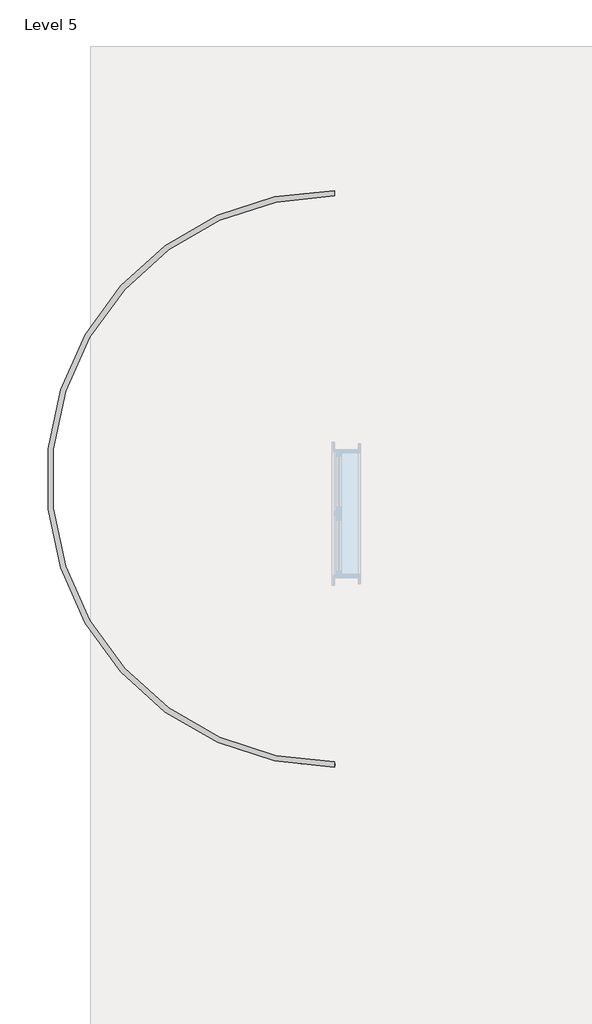
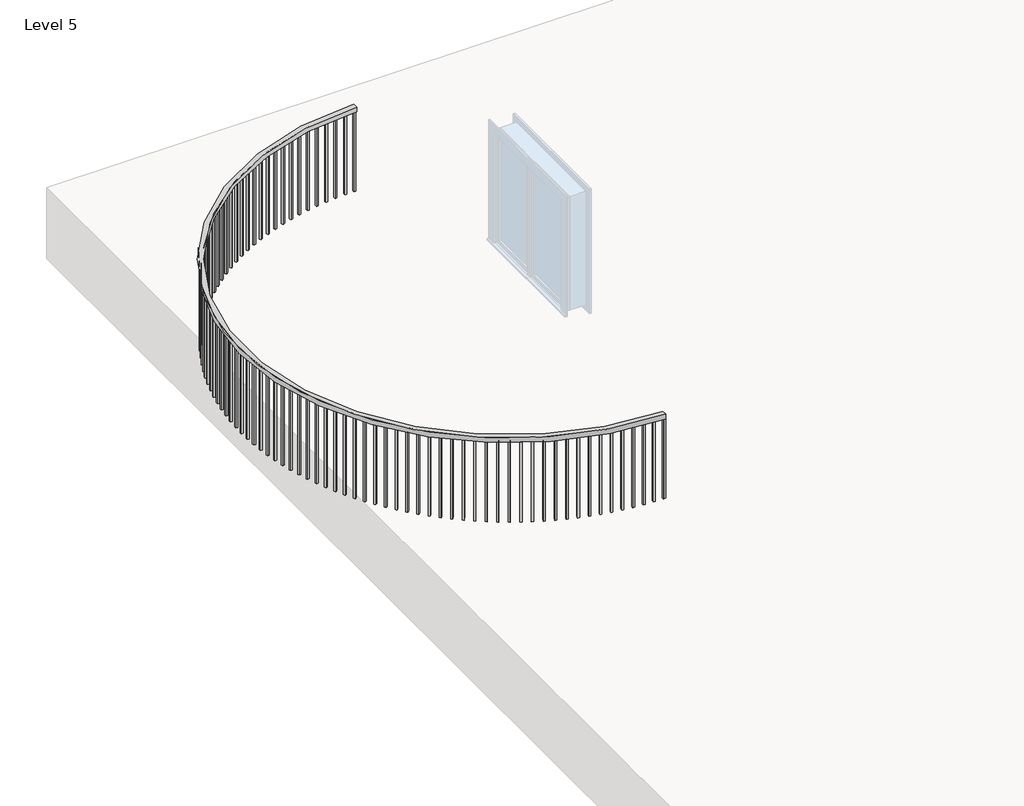
# One storey, part 2 of 2: 1 railing.
"""IFC4 building model written with IfcOpenShell, lengths in millimetres."""

from ifc_helpers import new_model, si_unit, point, frame, frame_2d, origin, place, context, project, spatial, polyline, circle_curve, trimmed, segment, composite_curve, outline, extrude, element, save

model = new_model("IFC4")

# Units and contexts
model_context = context("Model", 3, world=origin())
ifc_project = project(units=[si_unit("LENGTHUNIT", "METRE", prefix="MILLI")], contexts=[model_context])

# Site, building, storey
site = spatial("IfcSite", under=ifc_project)
building = spatial("IfcBuilding", under=site)
storey = spatial("IfcBuildingStorey", under=building, Name="Level 5", Elevation=12192.0)

# Railing
placement = place(None, origin())
element("IfcRailing", 1, ObjectType="Handrail - Rectangular", at=placement, inside=storey, context=model_context, shape_type="SweptSolid", body=[
    extrude(outline(composite_curve([segment(trimmed(circle_curve(frame_2d((-15728.6368919, 10326.9945075)), 2743.2), [point((-15728.6368919, 7583.7945075))], [point((-15728.6368919, 13070.1945075))], False, "CARTESIAN"), True, "CONTINUOUS"), segment(polyline([(-15728.6368919, 13070.1945075), (-15728.6368919, 13019.3945075)]), True, "CONTINUOUS"), segment(trimmed(circle_curve(frame_2d((-15728.6368919, 10326.9945075)), 2692.4), [point((-15728.6368919, 13019.3945075))], [point((-15728.6368919, 7634.5945075))], True, "CARTESIAN"), True, "CONTINUOUS"), segment(polyline([(-15728.6368919, 7634.5945075), (-15728.6368919, 7583.7945075)]), True, "CONTINUOUS")], self_intersect=False)), frame((0.0, 0.0, 13055.6), z_axis=(0.0, 0.0, 1.0), x_axis=(1.0, 0.0, 0.0)), (0.0, 0.0, 1.0), 50.8),
    extrude(outline(polyline([(-15741.9957848, 7599.6855919), (-15741.9690055, 7618.735573), (-15722.9190243, 7618.7087937), (-15722.9458036, 7599.6588126), (-15741.9957848, 7599.6855919)])), frame((0.0, 0.0, 12192.0), z_axis=(0.0, 0.0, 1.0), x_axis=(1.0, 0.0, 0.0)), (0.0, 0.0, 1.0), 863.6),
    extrude(outline(polyline([(-15843.9181793, 7602.0903613), (-15843.1794358, 7621.1260319), (-15824.1437651, 7620.3872884), (-15824.8825087, 7601.3516177), (-15843.9181793, 7602.0903613)])), frame((0.0, 0.0, 12192.0), z_axis=(0.0, 0.0, 1.0), x_axis=(1.0, 0.0, 0.0)), (0.0, 0.0, 1.0), 863.6),
    extrude(outline(polyline([(-15945.6794868, 7608.3027461), (-15944.2298113, 7627.297507), (-15925.2350504, 7625.8478315), (-15926.6847259, 7606.8530706), (-15945.6794868, 7608.3027461)])), frame((0.0, 0.0, 12192.0), z_axis=(0.0, 0.0, 1.0), x_axis=(1.0, 0.0, 0.0)), (0.0, 0.0, 1.0), 863.6),
    extrude(outline(polyline([(-16047.1375121, 7618.3140656), (-16044.9789303, 7637.2413746), (-16026.0516213, 7635.0827927), (-16028.2102032, 7616.1554838), (-16047.1375121, 7618.3140656)])), frame((0.0, 0.0, 12192.0), z_axis=(0.0, 0.0, 1.0), x_axis=(1.0, 0.0, 0.0)), (0.0, 0.0, 1.0), 863.6),
    extrude(outline(polyline([(-16148.150484, 7632.1103305), (-16145.2860122, 7650.9437397), (-16126.452603, 7648.0792678), (-16129.3170749, 7629.2458587), (-16148.150484, 7632.1103305)])), frame((0.0, 0.0, 12192.0), z_axis=(0.0, 0.0, 1.0), x_axis=(1.0, 0.0, 0.0)), (0.0, 0.0, 1.0), 863.6),
    extrude(outline(polyline([(-16248.5772532, 7649.6722628), (-16245.0108939, 7668.3854555), (-16226.2977012, 7664.8190963), (-16229.8640605, 7646.1059035), (-16248.5772532, 7649.6722628)])), frame((0.0, 0.0, 12192.0), z_axis=(0.0, 0.0, 1.0), x_axis=(1.0, 0.0, 0.0)), (0.0, 0.0, 1.0), 863.6),
    extrude(outline(polyline([(-16348.2774892, 7670.9753224), (-16344.014226, 7689.54215), (-16325.4473984, 7685.2788868), (-16329.7106616, 7666.7120592), (-16348.2774892, 7670.9753224)])), frame((0.0, 0.0, 12192.0), z_axis=(0.0, 0.0, 1.0), x_axis=(1.0, 0.0, 0.0)), (0.0, 0.0, 1.0), 863.6),
    extrude(outline(polyline([(-16447.1118772, 7695.9897418), (-16442.1576672, 7714.3842602), (-16423.7631489, 7709.4300502), (-16428.7173589, 7691.0355319), (-16447.1118772, 7695.9897418)])), frame((0.0, 0.0, 12192.0), z_axis=(0.0, 0.0, 1.0), x_axis=(1.0, 0.0, 0.0)), (0.0, 0.0, 1.0), 863.6),
    extrude(outline(polyline([(-16544.9423119, 7724.6805674), (-16539.3040779, 7742.8770731), (-16521.1075722, 7737.2388391), (-16526.7458062, 7719.0423334), (-16544.9423119, 7724.6805674)])), frame((0.0, 0.0, 12192.0), z_axis=(0.0, 0.0, 1.0), x_axis=(1.0, 0.0, 0.0)), (0.0, 0.0, 1.0), 863.6),
    extrude(outline(polyline([(-16641.632091, 7757.0077083), (-16635.3177115, 7774.9807746), (-16617.3446452, 7768.6663951), (-16623.6590247, 7750.6933288), (-16641.632091, 7757.0077083)])), frame((0.0, 0.0, 12192.0), z_axis=(0.0, 0.0, 1.0), x_axis=(1.0, 0.0, 0.0)), (0.0, 0.0, 1.0), 863.6),
    extrude(outline(polyline([(-16737.0461061, 7792.9259926), (-16730.0644044, 7810.6505051), (-16712.3398919, 7803.6688034), (-16719.3215936, 7785.9442909), (-16737.0461061, 7792.9259926)])), frame((0.0, 0.0, 12192.0), z_axis=(0.0, 0.0, 1.0), x_axis=(1.0, 0.0, 0.0)), (0.0, 0.0, 1.0), 863.6),
    extrude(outline(polyline([(-16831.0510314, 7832.3852302), (-16823.4117634, 7849.8364217), (-16805.9605719, 7842.1971536), (-16813.59984, 7824.7459621), (-16831.0510314, 7832.3852302)])), frame((0.0, 0.0, 12192.0), z_axis=(0.0, 0.0, 1.0), x_axis=(1.0, 0.0, 0.0)), (0.0, 0.0, 1.0), 863.6),
    extrude(outline(polyline([(-16923.5155103, 7875.3302832), (-16915.2293505, 7892.4837684), (-16898.0758652, 7884.1976086), (-16906.362025, 7867.0441234), (-16923.5155103, 7875.3302832)])), frame((0.0, 0.0, 12192.0), z_axis=(0.0, 0.0, 1.0), x_axis=(1.0, 0.0, 0.0)), (0.0, 0.0, 1.0), 863.6),
    extrude(outline(polyline([(-17014.3103383, 7921.7011427), (-17005.3888654, 7938.5329525), (-16988.5570556, 7929.6114796), (-16997.4785285, 7912.7796698), (-17014.3103383, 7921.7011427)])), frame((0.0, 0.0, 12192.0), z_axis=(0.0, 0.0, 1.0), x_axis=(1.0, 0.0, 0.0)), (0.0, 0.0, 1.0), 863.6),
    extrude(outline(polyline([(-17103.3086445, 7971.4330131), (-17093.7643247, 7987.9196276), (-17077.2777101, 7978.3753079), (-17086.8220299, 7961.8886933), (-17103.3086445, 7971.4330131)])), frame((0.0, 0.0, 12192.0), z_axis=(0.0, 0.0, 1.0), x_axis=(1.0, 0.0, 0.0)), (0.0, 0.0, 1.0), 863.6),
    extrude(outline(polyline([(-17190.3860679, 8024.4564019), (-17180.2322379, 8040.5747838), (-17164.1138559, 8030.4209539), (-17174.2676859, 8014.3025719), (-17190.3860679, 8024.4564019)])), frame((0.0, 0.0, 12192.0), z_axis=(0.0, 0.0, 1.0), x_axis=(1.0, 0.0, 0.0)), (0.0, 0.0, 1.0), 863.6),
    extrude(outline(polyline([(-17275.4209318, 8080.6972174), (-17264.67178, 8096.424844), (-17248.9441535, 8085.6756922), (-17259.6933053, 8069.9480657), (-17275.4209318, 8080.6972174)])), frame((0.0, 0.0, 12192.0), z_axis=(0.0, 0.0, 1.0), x_axis=(1.0, 0.0, 0.0)), (0.0, 0.0, 1.0), 863.6),
    extrude(outline(polyline([(-17358.2944137, 8140.0768723), (-17346.9649603, 8155.3917666), (-17331.6500661, 8144.0623132), (-17342.9795194, 8128.747419), (-17358.2944137, 8140.0768723)])), frame((0.0, 0.0, 12192.0), z_axis=(0.0, 0.0, 1.0), x_axis=(1.0, 0.0, 0.0)), (0.0, 0.0, 1.0), 863.6),
    extrude(outline(polyline([(-17438.8907113, 8202.512393), (-17426.9967874, 8217.3931549), (-17412.1160255, 8205.499231), (-17424.0099494, 8190.6184691), (-17438.8907113, 8202.512393)])), frame((0.0, 0.0, 12192.0), z_axis=(0.0, 0.0, 1.0), x_axis=(1.0, 0.0, 0.0)), (0.0, 0.0, 1.0), 863.6),
    extrude(outline(polyline([(-17517.0972041, 8267.9165359), (-17504.6554295, 8282.3423719), (-17490.2295935, 8269.9005973), (-17502.671368, 8255.4747613), (-17517.0972041, 8267.9165359)])), frame((0.0, 0.0, 12192.0), z_axis=(0.0, 0.0, 1.0), x_axis=(1.0, 0.0, 0.0)), (0.0, 0.0, 1.0), 863.6),
    extrude(outline(polyline([(-17592.8046111, 8336.1979092), (-17579.8323713, 8350.1486616), (-17565.8816189, 8337.1764217), (-17578.8538587, 8323.2256693), (-17592.8046111, 8336.1979092)])), frame((0.0, 0.0, 12192.0), z_axis=(0.0, 0.0, 1.0), x_axis=(1.0, 0.0, 0.0)), (0.0, 0.0, 1.0), 863.6),
    extrude(outline(polyline([(-17665.9071435, 8407.2611006), (-17652.422565, 8420.7172754), (-17638.9663901, 8407.2326969), (-17652.4509687, 8393.7765221), (-17665.9071435, 8407.2611006)])), frame((0.0, 0.0, 12192.0), z_axis=(0.0, 0.0, 1.0), x_axis=(1.0, 0.0, 0.0)), (0.0, 0.0, 1.0), 863.6),
    extrude(outline(polyline([(-17736.3026522, 8481.0068109), (-17722.3245775, 8493.9496053), (-17709.3817831, 8479.9715306), (-17723.3598578, 8467.0287361), (-17736.3026522, 8481.0068109)])), frame((0.0, 0.0, 12192.0), z_axis=(0.0, 0.0, 1.0), x_axis=(1.0, 0.0, 0.0)), (0.0, 0.0, 1.0), 863.6),
    extrude(outline(polyline([(-17803.8927708, 8557.3319921), (-17789.4407321, 8569.7433206), (-17777.0294035, 8555.2912819), (-17791.4814423, 8542.8799533), (-17803.8927708, 8557.3319921)])), frame((0.0, 0.0, 12192.0), z_axis=(0.0, 0.0, 1.0), x_axis=(1.0, 0.0, 0.0)), (0.0, 0.0, 1.0), 863.6),
    extrude(outline(polyline([(-17868.583053, 8636.1299922), (-17853.6772446, 8647.992512), (-17841.8147248, 8633.0867036), (-17856.7205331, 8621.2241838), (-17868.583053, 8636.1299922)])), frame((0.0, 0.0, 12192.0), z_axis=(0.0, 0.0, 1.0), x_axis=(1.0, 0.0, 0.0)), (0.0, 0.0, 1.0), 863.6),
    extrude(outline(polyline([(-17930.2831044, 8717.2907036), (-17914.9443548, 8728.5878387), (-17903.6472197, 8713.2490891), (-17918.9859693, 8701.951954), (-17930.2831044, 8717.2907036)])), frame((0.0, 0.0, 12192.0), z_axis=(0.0, 0.0, 1.0), x_axis=(1.0, 0.0, 0.0)), (0.0, 0.0, 1.0), 863.6),
    extrude(outline(polyline([(-17988.9067092, 8800.7007172), (-17973.1564519, 8811.4166817), (-17962.4404874, 8795.6664245), (-17978.1907447, 8784.9504599), (-17988.9067092, 8800.7007172)])), frame((0.0, 0.0, 12192.0), z_axis=(0.0, 0.0, 1.0), x_axis=(1.0, 0.0, 0.0)), (0.0, 0.0, 1.0), 863.6),
    extrude(outline(polyline([(-18044.3719504, 8886.2434811), (-18028.2321938, 8896.3633011), (-18018.1123738, 8880.2235446), (-18034.2521303, 8870.1037245), (-18044.3719504, 8886.2434811)])), frame((0.0, 0.0, 12192.0), z_axis=(0.0, 0.0, 1.0), x_axis=(1.0, 0.0, 0.0)), (0.0, 0.0, 1.0), 863.6),
    extrude(outline(polyline([(-18096.6013241, 8973.7994628), (-18080.094621, 8983.3089976), (-18070.5850862, 8966.8022945), (-18087.0917894, 8957.2927597), (-18096.6013241, 8973.7994628)])), frame((0.0, 0.0, 12192.0), z_axis=(0.0, 0.0, 1.0), x_axis=(1.0, 0.0, 0.0)), (0.0, 0.0, 1.0), 863.6),
    extrude(outline(polyline([(-18145.5218483, 9063.2463171), (-18128.6712641, 9072.1322785), (-18119.7853026, 9055.2816943), (-18136.6358868, 9046.3957328), (-18145.5218483, 9063.2463171)])), frame((0.0, 0.0, 12192.0), z_axis=(0.0, 0.0, 1.0), x_axis=(1.0, 0.0, 0.0)), (0.0, 0.0, 1.0), 863.6),
    extrude(outline(polyline([(-18191.0651643, 9154.4590562), (-18173.894245, 9162.7090277), (-18165.6442735, 9145.5381083), (-18182.8151929, 9137.2881369), (-18191.0651643, 9154.4590562)])), frame((0.0, 0.0, 12192.0), z_axis=(0.0, 0.0, 1.0), x_axis=(1.0, 0.0, 0.0)), (0.0, 0.0, 1.0), 863.6),
    extrude(outline(polyline([(-18233.1676328, 9247.3102252), (-18215.7003719, 9254.9126786), (-18208.0979185, 9237.4454177), (-18225.5651793, 9229.8429643), (-18233.1676328, 9247.3102252)])), frame((0.0, 0.0, 12192.0), z_axis=(0.0, 0.0, 1.0), x_axis=(1.0, 0.0, 0.0)), (0.0, 0.0, 1.0), 863.6),
    extrude(outline(polyline([(-18271.7704221, 9341.6700793), (-18254.0312274, 9348.6143915), (-18247.0869153, 9330.8751968), (-18264.82611, 9323.9308846), (-18271.7704221, 9341.6700793)])), frame((0.0, 0.0, 12192.0), z_axis=(0.0, 0.0, 1.0), x_axis=(1.0, 0.0, 0.0)), (0.0, 0.0, 1.0), 863.6),
    extrude(outline(polyline([(-18306.8195913, 9437.4067659), (-18288.8332504, 9443.6832333), (-18282.5567831, 9425.6968925), (-18300.5431239, 9419.4204251), (-18306.8195913, 9437.4067659)])), frame((0.0, 0.0, 12192.0), z_axis=(0.0, 0.0, 1.0), x_axis=(1.0, 0.0, 0.0)), (0.0, 0.0, 1.0), 863.6),
    extrude(outline(polyline([(-18338.2661646, 9534.3865084), (-18320.0578106, 9539.9863606), (-18314.4579584, 9521.7780066), (-18332.6663124, 9516.1781544), (-18338.2661646, 9534.3865084)])), frame((0.0, 0.0, 12192.0), z_axis=(0.0, 0.0, 1.0), x_axis=(1.0, 0.0, 0.0)), (0.0, 0.0, 1.0), 863.6),
    extrude(outline(polyline([(-18366.0662006, 9632.4737931), (-18347.6612768, 9637.3892053), (-18342.7458646, 9618.9842814), (-18361.1507885, 9614.0688692), (-18366.0662006, 9632.4737931)])), frame((0.0, 0.0, 12192.0), z_axis=(0.0, 0.0, 1.0), x_axis=(1.0, 0.0, 0.0)), (0.0, 0.0, 1.0), 863.6),
    extrude(outline(polyline([(-18390.1808532, 9731.5315588), (-18371.6050774, 9735.7556625), (-18367.3809737, 9717.1798866), (-18385.9567496, 9712.955783), (-18390.1808532, 9731.5315588)])), frame((0.0, 0.0, 12192.0), z_axis=(0.0, 0.0, 1.0), x_axis=(1.0, 0.0, 0.0)), (0.0, 0.0, 1.0), 863.6),
    extrude(outline(polyline([(-18410.576426, 9831.4213883), (-18391.8557549, 9834.9482809), (-18388.3288623, 9816.2276097), (-18407.0495335, 9812.7007171), (-18410.576426, 9831.4213883)])), frame((0.0, 0.0, 12192.0), z_axis=(0.0, 0.0, 1.0), x_axis=(1.0, 0.0, 0.0)), (0.0, 0.0, 1.0), 863.6),
    extrude(outline(polyline([(-18427.2244196, 9932.0037015), (-18408.3850122, 9934.8284548), (-18405.560259, 9915.9890475), (-18424.3996663, 9913.1642942), (-18427.2244196, 9932.0037015)])), frame((0.0, 0.0, 12192.0), z_axis=(0.0, 0.0, 1.0), x_axis=(1.0, 0.0, 0.0)), (0.0, 0.0, 1.0), 863.6),
    extrude(outline(polyline([(-18440.1015709, 10033.1379509), (-18421.1697524, 10035.2566177), (-18419.0510856, 10016.3247992), (-18437.9829041, 10014.2061324), (-18440.1015709, 10033.1379509)])), frame((0.0, 0.0, 12192.0), z_axis=(0.0, 0.0, 1.0), x_axis=(1.0, 0.0, 0.0)), (0.0, 0.0, 1.0), 863.6),
    extrude(outline(polyline([(-18449.1898863, 10134.6828176), (-18430.1921108, 10136.0924374), (-18428.782491, 10117.094662), (-18447.7802664, 10115.6850421), (-18449.1898863, 10134.6828176)])), frame((0.0, 0.0, 12192.0), z_axis=(0.0, 0.0, 1.0), x_axis=(1.0, 0.0, 0.0)), (0.0, 0.0, 1.0), 863.6),
    extrude(outline(polyline([(-18454.4766663, 10236.4964089), (-18435.4394802, 10237.1950121), (-18434.740877, 10218.157826), (-18453.7780631, 10217.4592228), (-18454.4766663, 10236.4964089)])), frame((0.0, 0.0, 12192.0), z_axis=(0.0, 0.0, 1.0), x_axis=(1.0, 0.0, 0.0)), (0.0, 0.0, 1.0), 863.6),
    extrude(outline(polyline([(-18455.9545234, 10338.4364568), (-18436.9045281, 10338.4230671), (-18436.9179178, 10319.3730718), (-18455.967913, 10319.3864615), (-18455.9545234, 10338.4364568)])), frame((0.0, 0.0, 12192.0), z_axis=(0.0, 0.0, 1.0), x_axis=(1.0, 0.0, 0.0)), (0.0, 0.0, 1.0), 863.6),
    extrude(outline(polyline([(-18453.6213926, 10440.3605163), (-18434.5852074, 10439.6351526), (-18435.3105712, 10420.5989673), (-18454.3467564, 10421.3243311), (-18453.6213926, 10440.3605163)])), frame((0.0, 0.0, 12192.0), z_axis=(0.0, 0.0, 1.0), x_axis=(1.0, 0.0, 0.0)), (0.0, 0.0, 1.0), 863.6),
    extrude(outline(polyline([(-18447.4805342, 10542.1261652), (-18428.4847591, 10540.6898408), (-18429.9210834, 10521.6940657), (-18448.9168585, 10523.13039), (-18447.4805342, 10542.1261652)])), frame((0.0, 0.0, 12192.0), z_axis=(0.0, 0.0, 1.0), x_axis=(1.0, 0.0, 0.0)), (0.0, 0.0, 1.0), 863.6),
    extrude(outline(polyline([(-18437.5405288, 10643.5912021), (-18418.6117074, 10641.4459242), (-18420.7569852, 10622.5171027), (-18439.6858067, 10624.6623806), (-18437.5405288, 10643.5912021)])), frame((0.0, 0.0, 12192.0), z_axis=(0.0, 0.0, 1.0), x_axis=(1.0, 0.0, 0.0)), (0.0, 0.0, 1.0), 863.6),
    extrude(outline(polyline([(-18423.8152662, 10744.613846), (-18404.9798483, 10741.7626123), (-18407.8310821, 10722.9271944), (-18426.6664999, 10725.7784281), (-18423.8152662, 10744.613846)])), frame((0.0, 0.0, 12192.0), z_axis=(0.0, 0.0, 1.0), x_axis=(1.0, 0.0, 0.0)), (0.0, 0.0, 1.0), 863.6),
    extrude(outline(polyline([(-18406.3239251, 10845.0529341), (-18387.6082304, 10841.4997286), (-18391.1614358, 10822.7840338), (-18409.8771306, 10826.3372393), (-18406.3239251, 10845.0529341)])), frame((0.0, 0.0, 12192.0), z_axis=(0.0, 0.0, 1.0), x_axis=(1.0, 0.0, 0.0)), (0.0, 0.0, 1.0), 863.6),
    extrude(outline(polyline([(-18385.0909469, 10944.7681188), (-18366.5211274, 10940.5179066), (-18370.7713395, 10921.9480871), (-18389.341159, 10926.1982992), (-18385.0909469, 10944.7681188)])), frame((0.0, 0.0, 12192.0), z_axis=(0.0, 0.0, 1.0), x_axis=(1.0, 0.0, 0.0)), (0.0, 0.0, 1.0), 863.6),
    extrude(outline(polyline([(-18360.1460013, 11043.6200641), (-18341.7480054, 11038.6787843), (-18346.6892852, 11020.2807884), (-18365.0872811, 11025.2220682), (-18360.1460013, 11043.6200641)])), frame((0.0, 0.0, 12192.0), z_axis=(0.0, 0.0, 1.0), x_axis=(1.0, 0.0, 0.0)), (0.0, 0.0, 1.0), 863.6),
    extrude(outline(polyline([(-18331.5239448, 11141.4706405), (-18313.3234807, 11135.8451977), (-18318.9489235, 11117.6447336), (-18337.1493876, 11123.2701765), (-18331.5239448, 11141.4706405)])), frame((0.0, 0.0, 12192.0), z_axis=(0.0, 0.0, 1.0), x_axis=(1.0, 0.0, 0.0)), (0.0, 0.0, 1.0), 863.6),
    extrude(outline(polyline([(-18299.2647721, 11238.1831175), (-18281.287272, 11231.8813723), (-18287.5890173, 11213.9038722), (-18305.5665173, 11220.2056175), (-18299.2647721, 11238.1831175)])), frame((0.0, 0.0, 12192.0), z_axis=(0.0, 0.0, 1.0), x_axis=(1.0, 0.0, 0.0)), (0.0, 0.0, 1.0), 863.6),
    extrude(outline(polyline([(-18263.4135602, 11333.6223549), (-18245.6841449, 11326.6531129), (-18252.6533869, 11308.9236976), (-18270.3828021, 11315.8929396), (-18263.4135602, 11333.6223549)])), frame((0.0, 0.0, 12192.0), z_axis=(0.0, 0.0, 1.0), x_axis=(1.0, 0.0, 0.0)), (0.0, 0.0, 1.0), 863.6),
    extrude(outline(polyline([(-18224.0204055, 11427.6549917), (-18206.5638489, 11420.0279914), (-18214.1908492, 11402.5714348), (-18231.6474057, 11410.1984351), (-18224.0204055, 11427.6549917)])), frame((0.0, 0.0, 12192.0), z_axis=(0.0, 0.0, 1.0), x_axis=(1.0, 0.0, 0.0)), (0.0, 0.0, 1.0), 863.6),
    extrude(outline(polyline([(-18181.1403535, 11520.1496324), (-18163.9810484, 11511.8755313), (-18172.2551495, 11494.7162262), (-18189.4144546, 11502.9903273), (-18181.1403535, 11520.1496324)])), frame((0.0, 0.0, 12192.0), z_axis=(0.0, 0.0, 1.0), x_axis=(1.0, 0.0, 0.0)), (0.0, 0.0, 1.0), 863.6),
    extrude(outline(polyline([(-18134.8333222, 11610.9770307), (-18117.995246, 11602.0673905), (-18126.9048862, 11585.2293142), (-18143.7429624, 11594.1389544), (-18134.8333222, 11610.9770307)])), frame((0.0, 0.0, 12192.0), z_axis=(0.0, 0.0, 1.0), x_axis=(1.0, 0.0, 0.0)), (0.0, 0.0, 1.0), 863.6),
    extrude(outline(polyline([(-18085.1640183, 11700.0102698), (-18068.6706994, 11690.4775403), (-18078.2034289, 11673.9842214), (-18094.6967478, 11683.5169509), (-18085.1640183, 11700.0102698)])), frame((0.0, 0.0, 12192.0), z_axis=(0.0, 0.0, 1.0), x_axis=(1.0, 0.0, 0.0)), (0.0, 0.0, 1.0), 863.6),
    extrude(outline(polyline([(-18032.2018467, 11787.1249402), (-18016.0763318, 11776.9824419), (-18026.2188302, 11760.8569271), (-18042.344345, 11770.9994254), (-18032.2018467, 11787.1249402)])), frame((0.0, 0.0, 12192.0), z_axis=(0.0, 0.0, 1.0), x_axis=(1.0, 0.0, 0.0)), (0.0, 0.0, 1.0), 863.6),
    extrude(outline(polyline([(-17976.0208133, 11872.199313), (-17960.2856354, 11861.4612184), (-17971.0237301, 11845.7260405), (-17986.758908, 11856.4641351), (-17976.0208133, 11872.199313)])), frame((0.0, 0.0, 12192.0), z_axis=(0.0, 0.0, 1.0), x_axis=(1.0, 0.0, 0.0)), (0.0, 0.0, 1.0), 863.6),
    extrude(outline(polyline([(-17916.6994223, 11955.1145106), (-17901.3765687, 11943.7958244), (-17912.6952549, 11928.4729708), (-17928.0181085, 11939.791657), (-17916.6994223, 11955.1145106)])), frame((0.0, 0.0, 12192.0), z_axis=(0.0, 0.0, 1.0), x_axis=(1.0, 0.0, 0.0)), (0.0, 0.0, 1.0), 863.6),
    extrude(outline(polyline([(-17854.3205656, 12035.7546722), (-17839.4314475, 12023.8712105), (-17851.3149093, 12008.9820924), (-17866.2040274, 12020.8655541), (-17854.3205656, 12035.7546722)])), frame((0.0, 0.0, 12192.0), z_axis=(0.0, 0.0, 1.0), x_axis=(1.0, 0.0, 0.0)), (0.0, 0.0, 1.0), 863.6),
    extrude(outline(polyline([(-17788.9714078, 12114.0071162), (-17774.5368304, 12101.5754842), (-17786.9684624, 12087.1409068), (-17801.4030399, 12099.5725388), (-17788.9714078, 12114.0071162)])), frame((0.0, 0.0, 12192.0), z_axis=(0.0, 0.0, 1.0), x_axis=(1.0, 0.0, 0.0)), (0.0, 0.0, 1.0), 863.6),
    extrude(outline(polyline([(-17720.7432638, 12189.7624974), (-17706.783397, 12176.8000663), (-17719.7458282, 12162.8401996), (-17733.7056949, 12175.8026307), (-17720.7432638, 12189.7624974)])), frame((0.0, 0.0, 12192.0), z_axis=(0.0, 0.0, 1.0), x_axis=(1.0, 0.0, 0.0)), (0.0, 0.0, 1.0), 863.6),
    extrude(outline(polyline([(-17649.7314714, 12262.9149599), (-17636.265822, 12249.4398426), (-17649.7409393, 12235.9741932), (-17663.2065887, 12249.4493105), (-17649.7314714, 12262.9149599)])), frame((0.0, 0.0, 12192.0), z_axis=(0.0, 0.0, 1.0), x_axis=(1.0, 0.0, 0.0)), (0.0, 0.0, 1.0), 863.6),
    extrude(outline(polyline([(-17576.0352582, 12333.3622847), (-17563.0826422, 12319.3933106), (-17577.0516164, 12306.4406946), (-17590.0042323, 12320.4096688), (-17576.0352582, 12333.3622847)])), frame((0.0, 0.0, 12192.0), z_axis=(0.0, 0.0, 1.0), x_axis=(1.0, 0.0, 0.0)), (0.0, 0.0, 1.0), 863.6),
    extrude(outline(polyline([(-17499.7576028, 12401.0060332), (-17487.3361194, 12386.5627216), (-17501.779431, 12374.1412382), (-17514.2009144, 12388.5845499), (-17499.7576028, 12401.0060332)])), frame((0.0, 0.0, 12192.0), z_axis=(0.0, 0.0, 1.0), x_axis=(1.0, 0.0, 0.0)), (0.0, 0.0, 1.0), 863.6),
    extrude(outline(polyline([(-17421.0050909, 12465.751684), (-17409.1320972, 12450.8542171), (-17424.0295641, 12438.9812234), (-17435.9025578, 12453.8786903), (-17421.0050909, 12465.751684)])), frame((0.0, 0.0, 12192.0), z_axis=(0.0, 0.0, 1.0), x_axis=(1.0, 0.0, 0.0)), (0.0, 0.0, 1.0), 863.6),
    extrude(outline(polyline([(-17339.8877666, 12527.5087656), (-17328.5798531, 12512.1779602), (-17343.9106585, 12500.8700467), (-17355.218572, 12516.2008521), (-17339.8877666, 12527.5087656)])), frame((0.0, 0.0, 12192.0), z_axis=(0.0, 0.0, 1.0), x_axis=(1.0, 0.0, 0.0)), (0.0, 0.0, 1.0), 863.6),
    extrude(outline(polyline([(-17256.5189783, 12586.1909822), (-17245.791946, 12570.4482607), (-17261.5346675, 12559.7212285), (-17272.2616997, 12575.46395), (-17256.5189783, 12586.1909822)])), frame((0.0, 0.0, 12192.0), z_axis=(0.0, 0.0, 1.0), x_axis=(1.0, 0.0, 0.0)), (0.0, 0.0, 1.0), 863.6),
    extrude(outline(polyline([(-17171.0152203, 12641.716335), (-17160.8840587, 12625.5836953), (-17177.0166983, 12615.4525337), (-17187.14786, 12631.5851733), (-17171.0152203, 12641.716335)])), frame((0.0, 0.0, 12192.0), z_axis=(0.0, 0.0, 1.0), x_axis=(1.0, 0.0, 0.0)), (0.0, 0.0, 1.0), 863.6),
    extrude(outline(polyline([(-17083.4959706, 12694.0072362), (-17073.9748361, 12677.5072211), (-17090.4748512, 12667.9860867), (-17099.9959857, 12684.4861018), (-17083.4959706, 12694.0072362)])), frame((0.0, 0.0, 12192.0), z_axis=(0.0, 0.0, 1.0), x_axis=(1.0, 0.0, 0.0)), (0.0, 0.0, 1.0), 863.6),
    extrude(outline(polyline([(-16994.0835232, 12742.9906177), (-16985.1857201, 12726.1462833), (-17002.0300546, 12717.2484803), (-17010.9278576, 12734.0928147), (-16994.0835232, 12742.9906177)])), frame((0.0, 0.0, 12192.0), z_axis=(0.0, 0.0, 1.0), x_axis=(1.0, 0.0, 0.0)), (0.0, 0.0, 1.0), 863.6),
    extrude(outline(polyline([(-16902.9028175, 12788.5980331), (-16894.6407792, 12771.4329166), (-16911.8058957, 12763.1708783), (-16920.067934, 12780.3359948), (-16902.9028175, 12788.5980331)])), frame((0.0, 0.0, 12192.0), z_axis=(0.0, 0.0, 1.0), x_axis=(1.0, 0.0, 0.0)), (0.0, 0.0, 1.0), 863.6),
    extrude(outline(polyline([(-16810.081264, 12830.7657533), (-16802.4665353, 12813.3038403), (-16819.9284483, 12805.6891115), (-16827.543177, 12823.1510246), (-16810.081264, 12830.7657533)])), frame((0.0, 0.0, 12192.0), z_axis=(0.0, 0.0, 1.0), x_axis=(1.0, 0.0, 0.0)), (0.0, 0.0, 1.0), 863.6),
    extrude(outline(polyline([(-16715.7485659, 12869.4348557), (-16708.7917871, 12851.7005464), (-16726.5260965, 12844.7437676), (-16733.4828752, 12862.4780769), (-16715.7485659, 12869.4348557)])), frame((0.0, 0.0, 12192.0), z_axis=(0.0, 0.0, 1.0), x_axis=(1.0, 0.0, 0.0)), (0.0, 0.0, 1.0), 863.6),
    extrude(outline(polyline([(-16620.0365379, 12904.5513065), (-16613.74743, 12886.5693817), (-16631.7293549, 12880.2802738), (-16638.0184627, 12898.2621987), (-16620.0365379, 12904.5513065)])), frame((0.0, 0.0, 12192.0), z_axis=(0.0, 0.0, 1.0), x_axis=(1.0, 0.0, 0.0)), (0.0, 0.0, 1.0), 863.6),
    extrude(outline(polyline([(-16523.0789222, 12936.0660362), (-16517.4662733, 12917.8616226), (-16535.6706868, 12912.2489737), (-16541.2833357, 12930.4533872), (-16523.0789222, 12936.0660362)])), frame((0.0, 0.0, 12192.0), z_axis=(0.0, 0.0, 1.0), x_axis=(1.0, 0.0, 0.0)), (0.0, 0.0, 1.0), 863.6),
    extrude(outline(polyline([(-16425.0112015, 12963.9350078), (-16420.0828543, 12945.5335433), (-16438.4843187, 12940.6051961), (-16443.4126659, 12959.0066606), (-16425.0112015, 12963.9350078)])), frame((0.0, 0.0, 12192.0), z_axis=(0.0, 0.0, 1.0), x_axis=(1.0, 0.0, 0.0)), (0.0, 0.0, 1.0), 863.6),
    extrude(outline(polyline([(-16325.9704097, 12988.119279), (-16321.7332507, 12969.5464768), (-16340.306053, 12965.3093178), (-16344.5432119, 12983.8821201), (-16325.9704097, 12988.119279)])), frame((0.0, 0.0, 12192.0), z_axis=(0.0, 0.0, 1.0), x_axis=(1.0, 0.0, 0.0)), (0.0, 0.0, 1.0), 863.6),
    extrude(outline(polyline([(-16226.0949403, 13008.5850563), (-16222.5548904, 12989.8668687), (-16241.273078, 12986.3268188), (-16244.8131279, 13005.0450064), (-16226.0949403, 13008.5850563)])), frame((0.0, 0.0, 12192.0), z_axis=(0.0, 0.0, 1.0), x_axis=(1.0, 0.0, 0.0)), (0.0, 0.0, 1.0), 863.6),
    extrude(outline(polyline([(-16125.5243533, 13025.3037418), (-16122.686359, 13006.4663246), (-16141.5237763, 13003.6283304), (-16144.3617705, 13022.4657476), (-16125.5243533, 13025.3037418)])), frame((0.0, 0.0, 12192.0), z_axis=(0.0, 0.0, 1.0), x_axis=(1.0, 0.0, 0.0)), (0.0, 0.0, 1.0), 863.6),
    extrude(outline(polyline([(-16024.3991798, 13038.2519741), (-16022.2672069, 13019.3216494), (-16041.1975316, 13017.1896766), (-16043.3295045, 13036.1200012), (-16024.3991798, 13038.2519741)])), frame((0.0, 0.0, 12192.0), z_axis=(0.0, 0.0, 1.0), x_axis=(1.0, 0.0, 0.0)), (0.0, 0.0, 1.0), 863.6),
    extrude(outline(polyline([(-15922.8607261, 13047.41166), (-15921.4377537, 13028.41488), (-15940.4345336, 13026.9919075), (-15941.8575061, 13045.9886875), (-15922.8607261, 13047.41166)])), frame((0.0, 0.0, 12192.0), z_axis=(0.0, 0.0, 1.0), x_axis=(1.0, 0.0, 0.0)), (0.0, 0.0, 1.0), 863.6),
    extrude(outline(polyline([(-15821.0508759, 13052.7700002), (-15820.3388922, 13033.7333099), (-15839.3755825, 13033.0213262), (-15840.0875662, 13052.0580165), (-15821.0508759, 13052.7700002)])), frame((0.0, 0.0, 12192.0), z_axis=(0.0, 0.0, 1.0), x_axis=(1.0, 0.0, 0.0)), (0.0, 0.0, 1.0), 863.6),
    extrude(outline(polyline([(-15747.7201959, 7599.7196389), (-15747.653432, 7618.7695219), (-15728.603549, 7618.702758), (-15728.6703128, 7599.652875), (-15747.7201959, 7599.7196389)])), frame((0.0, 0.0, 12192.0), z_axis=(0.0, 0.0, 1.0), x_axis=(1.0, 0.0, 0.0)), (0.0, 0.0, 1.0), 863.6),
    extrude(outline(polyline([(-15728.6703128, 13054.3361399), (-15728.603549, 13035.2862569), (-15747.653432, 13035.219493), (-15747.7201959, 13054.2693761), (-15728.6703128, 13054.3361399)])), frame((0.0, 0.0, 12192.0), z_axis=(0.0, 0.0, 1.0), x_axis=(1.0, 0.0, 0.0)), (0.0, 0.0, 1.0), 863.6),
])

save(model, "model.ifc")

# Revit data of these elements
# Type "Handrail - Rectangular"
#   Assembly Code = "C2010400"
#   built-in parameter 1008612 = 0.0416667 (stored number, unit not read)
#   built-in parameter 1008611 = 0.0416667 (stored number, unit not read)
#   built-in parameter 1008609 = 0.333333 (stored number, unit not read)
#   built-in parameter 1008604 = 0.166667 (stored number, unit not read)
#   built-in parameter 1008603 = 0.166667 (stored number, unit not read)
#   Railing Height = 3' - 0"
#   built-in parameter 1008630 = 2
#   built-in parameter 1008610 = 2
#   built-in parameter 1008618 = Baluster - Square : 3/4"
# Element 1 (IfcRailing, "Handrail - Rectangular")
#   Phase Created = New Construction
